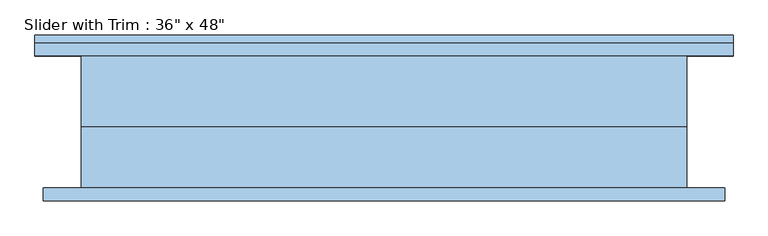
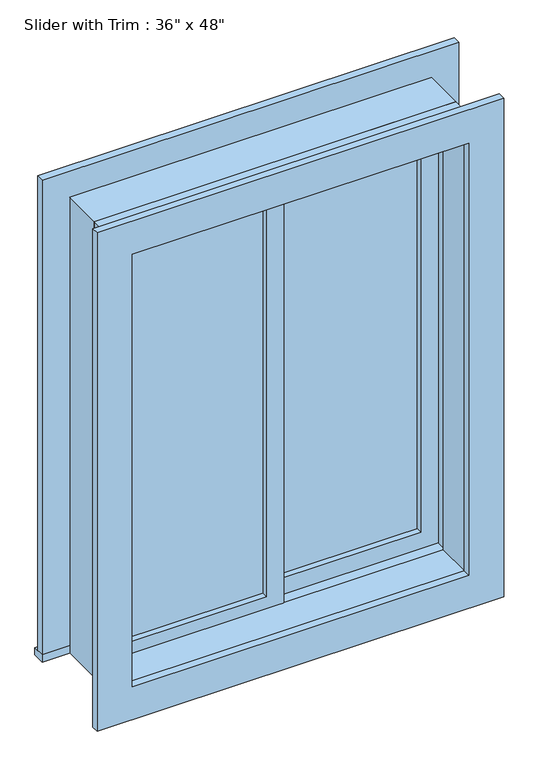
"""IFC4 building model written with IfcOpenShell, lengths in millimetres: window geometry."""

from ifc_helpers import new_model, si_unit, frame, origin, place, context, project, spatial, polyline, outline, extrude, source, transform, mapped, element, save


def window_242facca(model_context):
    return source(origin(), model_context, "Body", "SweptSolid", [
        extrude(outline(polyline([(-393.7, 20.625), (-22.225, 20.625), (-22.225, 7.925), (-393.7, 7.925), (-393.7, 20.625)])), frame((0.0, 0.0, 977.9), z_axis=(0.0, 0.0, 1.0), x_axis=(1.0, 0.0, 0.0)), (0.0, 0.0, 1.0), 1092.2),
        extrude(outline(polyline([(2114.55, -438.15), (933.45, -438.15), (933.45, 22.225), (2114.55, 22.225), (2114.55, -438.15)]), holes=[polyline([(2070.1, -393.7), (2070.1, -22.225), (977.9, -22.225), (977.9, -393.7), (2070.1, -393.7)])]), frame((0.0, -7.95, 0.0), z_axis=(0.0, 1.0, 0.0), x_axis=(0.0, 0.0, 1.0)), (0.0, 0.0, 1.0), 44.45),
        extrude(outline(polyline([(-527.05, 131.75), (527.05, 131.75), (527.05, 100.0), (-527.05, 100.0), (-527.05, 131.75)])), frame((0.0, 0.0, 914.4), z_axis=(0.0, 0.0, 1.0), x_axis=(1.0, 0.0, 0.0)), (0.0, 0.0, 1.0), 19.05),
        extrude(outline(polyline([(2114.55, -438.15), (2114.55, 438.15), (933.45, 438.15), (933.45, 527.05), (2203.45, 527.05), (2203.45, -527.05), (933.45, -527.05), (933.45, -438.15), (2114.55, -438.15)])), frame((0.0, 100.0, 0.0), z_axis=(0.0, 1.0, 0.0), x_axis=(0.0, 0.0, 1.0)), (0.0, 0.0, 1.0), 19.05),
        extrude(outline(polyline([(2190.75, 514.35), (2190.75, -514.35), (857.25, -514.35), (857.25, 514.35), (2190.75, 514.35)]), holes=[polyline([(2101.85, 425.45), (946.15, 425.45), (946.15, -425.45), (2101.85, -425.45), (2101.85, 425.45)])]), frame((0.0, -119.05, 0.0), z_axis=(0.0, 1.0, 0.0), x_axis=(0.0, 0.0, 1.0)), (0.0, 0.0, 1.0), 19.05),
        extrude(outline(polyline([(393.7, 52.375), (22.225, 52.375), (22.225, 65.075), (393.7, 65.075), (393.7, 52.375)])), frame((0.0, 0.0, 977.9), z_axis=(0.0, 0.0, 1.0), x_axis=(1.0, 0.0, 0.0)), (0.0, 0.0, 1.0), 1092.2),
        extrude(outline(polyline([(2114.55, -22.225), (933.45, -22.225), (933.45, 438.15), (2114.55, 438.15), (2114.55, -22.225)]), holes=[polyline([(2070.1, 22.225), (2070.1, 393.7), (977.9, 393.7), (977.9, 22.225), (2070.1, 22.225)])]), frame((0.0, 36.5, 0.0), z_axis=(0.0, 1.0, 0.0), x_axis=(0.0, 0.0, 1.0)), (0.0, 0.0, 1.0), 44.45),
        extrude(outline(polyline([(2133.6, -457.2), (914.4, -457.2), (914.4, 457.2), (2133.6, 457.2), (2133.6, -457.2)]), holes=[polyline([(2101.85, -425.45), (2101.85, 425.45), (946.15, 425.45), (946.15, -425.45), (2101.85, -425.45)])]), frame((0.0, -100.0, 0.0), z_axis=(0.0, 1.0, 0.0), x_axis=(0.0, 0.0, 1.0)), (0.0, 0.0, 1.0), 92.05),
        extrude(outline(polyline([(2133.6, 457.2), (2133.6, -457.2), (914.4, -457.2), (914.4, 457.2), (2133.6, 457.2)]), holes=[polyline([(2114.55, 438.15), (933.45, 438.15), (933.45, -438.15), (2114.55, -438.15), (2114.55, 438.15)])]), frame((0.0, -7.95, 0.0), z_axis=(0.0, 1.0, 0.0), x_axis=(0.0, 0.0, 1.0)), (0.0, 0.0, 1.0), 107.95),
    ])


if __name__ == "__main__":
    model = new_model("IFC4")
    model_context = context("Model", 3, world=origin())
    ifc_project = project(units=[si_unit("LENGTHUNIT", "METRE", prefix="MILLI")], contexts=[model_context])
    site = spatial("IfcSite", under=ifc_project)
    building = spatial("IfcBuilding", under=site)
    placement = place(None, origin())
    window_shape = window_242facca(model_context)
    element("IfcWindow", 1, ObjectType="Slider with Trim : 36\" x 48\"", at=placement, inside=building, context=model_context, shape_type="MappedRepresentation", body=[
        mapped(window_shape, transform((0.0, 0.0, 0.0), x_axis=(1.0, 0.0, 0.0), y_axis=(0.0, 1.0, 0.0), z_axis=(0.0, 0.0, 1.0))),
    ])
    save(model, "model.ifc")

# Revit data of these elements
# Type "Slider with Trim : 36\" x 48\""
#   Type Mark = "19"
#   Construction Type Id = "GSP4R"
#   Assembly Code = "B2020100"
#   Analytic Construction = "1/8 in Pilkington single glazing"
#   Visual Light Transmittance = 0.9
#   Solar Heat Gain Coefficient = 0.78
#   Heat Transfer Coefficient (U) = 3.6886 W/(m²·K)
#   Height = 4' - 0"
#   Default Sill Height = 3' - 0"
#   Trim Projection - Ext. = 0' - 0 3/4"
#   Trim Projection - Int. = 0' - 0 3/4"
#   Trim Width - Exterior = 0' - 3 1/2"
#   Trim Width - Interior = 0' - 3 1/2"
#   Width = 3' - 0"
#   Window Inset = 0' - 0 3/4"
#   Define Thermal Properties by = 1
#   Glass Pane Material = Glass
#   Sash Material = Sash
#   Trim Exterior Material = Trim
#   Trim Interior Material = Trim
#   Wall Closure = (empty or 0)
# Element 1 (IfcWindow, "Slider with Trim : 36\" x 48\"")
#   Materials on its faces: "Sash", "Trim", "Glass"
# Materials
#   "Glass": class "Glass", colour RGB 218 227 224, transparency 0.85, Description = "Soda Lime Glass", Cost = 0
#   "Sash": class "Wood", colour RGB 136 99 55, transparency 0
#   "Trim": class "Wood", colour RGB 224 178 126, transparency 0
